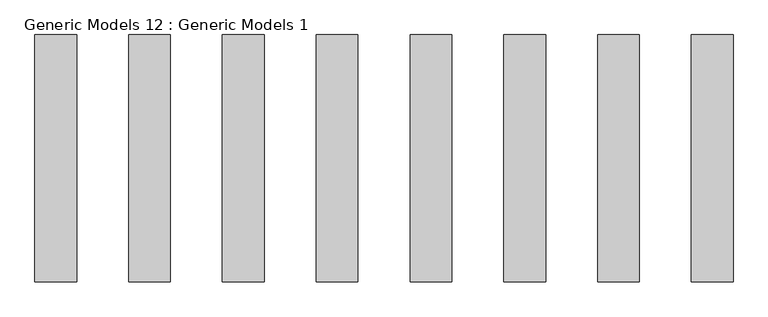
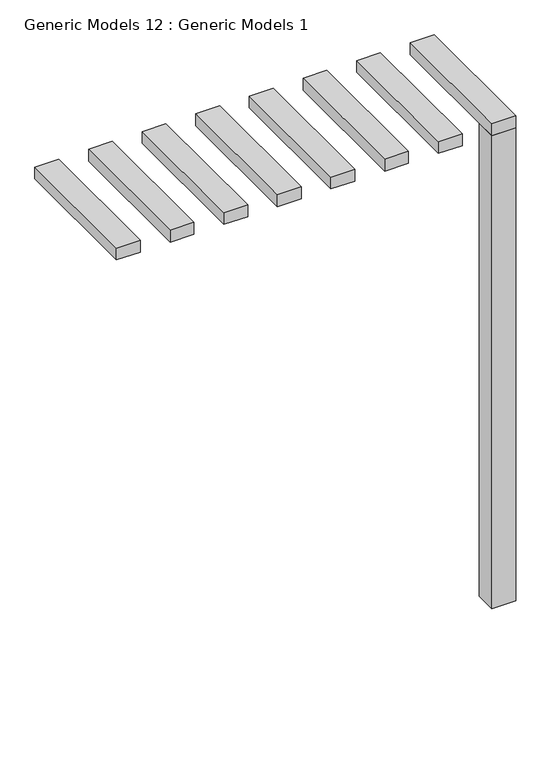
"""IFC4 building model written with IfcOpenShell, lengths in millimetres: proxy geometry, Generic Models 12 : Generic Models 1."""

from ifc_helpers import new_model, si_unit, frame, origin, origin_with_axes, place, context, project, spatial, polyline, outline, extrude, source, transform, mapped, element, save


def generic_models_12_generic_models_1_bdc4cd0d(model_context):
    return source(origin(), model_context, "Body", "SweptSolid", [
        extrude(outline(polyline([(-12100.1536806, -4709.7273102), (-11947.7536806, -4709.7273102), (-11947.7536806, -5613.7098142), (-12100.1536806, -5613.7098142), (-12100.1536806, -4709.7273102)])), frame((0.0, 0.0, 3200.4), z_axis=(0.0, 0.0, 1.0), x_axis=(1.0, 0.0, 0.0)), (0.0, 0.0, 1.0), 79.9931522),
        extrude(outline(polyline([(-11757.069475, -4709.7273102), (-11604.669475, -4709.7273102), (-11604.669475, -5613.7098142), (-11757.069475, -5613.7098142), (-11757.069475, -4709.7273102)])), frame((0.0, 0.0, 3200.4), z_axis=(0.0, 0.0, 1.0), x_axis=(1.0, 0.0, 0.0)), (0.0, 0.0, 1.0), 79.9931522),
        extrude(outline(polyline([(-11413.9852694, -4709.7273102), (-11261.5852694, -4709.7273102), (-11261.5852694, -5613.7098142), (-11413.9852694, -5613.7098142), (-11413.9852694, -4709.7273102)])), frame((0.0, 0.0, 3200.4), z_axis=(0.0, 0.0, 1.0), x_axis=(1.0, 0.0, 0.0)), (0.0, 0.0, 1.0), 79.9931522),
        extrude(outline(polyline([(-11070.9010638, -4709.7273102), (-10918.5010638, -4709.7273102), (-10918.5010638, -5613.7098142), (-11070.9010638, -5613.7098142), (-11070.9010638, -4709.7273102)])), frame((0.0, 0.0, 3200.4), z_axis=(0.0, 0.0, 1.0), x_axis=(1.0, 0.0, 0.0)), (0.0, 0.0, 1.0), 79.9931522),
        extrude(outline(polyline([(-10727.8168582, -4709.7273102), (-10575.4168582, -4709.7273102), (-10575.4168582, -5613.7098142), (-10727.8168582, -5613.7098142), (-10727.8168582, -4709.7273102)])), frame((0.0, 0.0, 3200.4), z_axis=(0.0, 0.0, 1.0), x_axis=(1.0, 0.0, 0.0)), (0.0, 0.0, 1.0), 79.9931522),
        extrude(outline(polyline([(-10384.7326527, -4709.7273102), (-10232.3326527, -4709.7273102), (-10232.3326527, -5613.7098142), (-10384.7326527, -5613.7098142), (-10384.7326527, -4709.7273102)])), frame((0.0, 0.0, 3200.4), z_axis=(0.0, 0.0, 1.0), x_axis=(1.0, 0.0, 0.0)), (0.0, 0.0, 1.0), 79.9931522),
        extrude(outline(polyline([(-10041.6484471, -4709.7273102), (-9889.2484471, -4709.7273102), (-9889.2484471, -5613.7098142), (-10041.6484471, -5613.7098142), (-10041.6484471, -4709.7273102)])), frame((0.0, 0.0, 3200.4), z_axis=(0.0, 0.0, 1.0), x_axis=(1.0, 0.0, 0.0)), (0.0, 0.0, 1.0), 79.9931522),
        extrude(outline(polyline([(-9698.5642415, -4709.7273102), (-9546.1642415, -4709.7273102), (-9546.1642415, -5613.7098142), (-9698.5642415, -5613.7098142), (-9698.5642415, -4709.7273102)])), frame((0.0, 0.0, 3200.4), z_axis=(0.0, 0.0, 1.0), x_axis=(1.0, 0.0, 0.0)), (0.0, 0.0, 1.0), 79.9931522),
        extrude(outline(polyline([(-9698.5642415, -5471.7273102), (-9546.1642415, -5471.7273102), (-9546.1642415, -5613.7098142), (-9698.5642415, -5613.7098142), (-9698.5642415, -5471.7273102)])), origin_with_axes(), (0.0, 0.0, 1.0), 3200.4),
    ])


if __name__ == "__main__":
    model = new_model("IFC4")
    model_context = context("Model", 3, world=origin())
    ifc_project = project(units=[si_unit("LENGTHUNIT", "METRE", prefix="MILLI")], contexts=[model_context])
    site = spatial("IfcSite", under=ifc_project)
    building = spatial("IfcBuilding", under=site)
    placement = place(None, origin())
    generic_models_12_generic_models_1_shape = generic_models_12_generic_models_1_bdc4cd0d(model_context)
    element("IfcBuildingElementProxy", 1, Name="Generic Models 12 : Generic Models 1", ObjectType="Generic Models 12 : Generic Models 1", at=placement, inside=building, context=model_context, shape_type="MappedRepresentation", body=[
        mapped(generic_models_12_generic_models_1_shape, transform((0.0, 0.0, 0.0), x_axis=(1.0, 0.0, 0.0), y_axis=(0.0, 1.0, 0.0), z_axis=(0.0, 0.0, 1.0))),
    ])
    save(model, "model.ifc")

# Revit data of these elements
# Element 1 (IfcBuildingElementProxy, "Generic Models 12 : Generic Models 1")
#   Materials on its faces: "exterior wall"
# Materials
#   "exterior wall": class "Generic", colour RGB 215 217 121, transparency 0, Cost = 0
